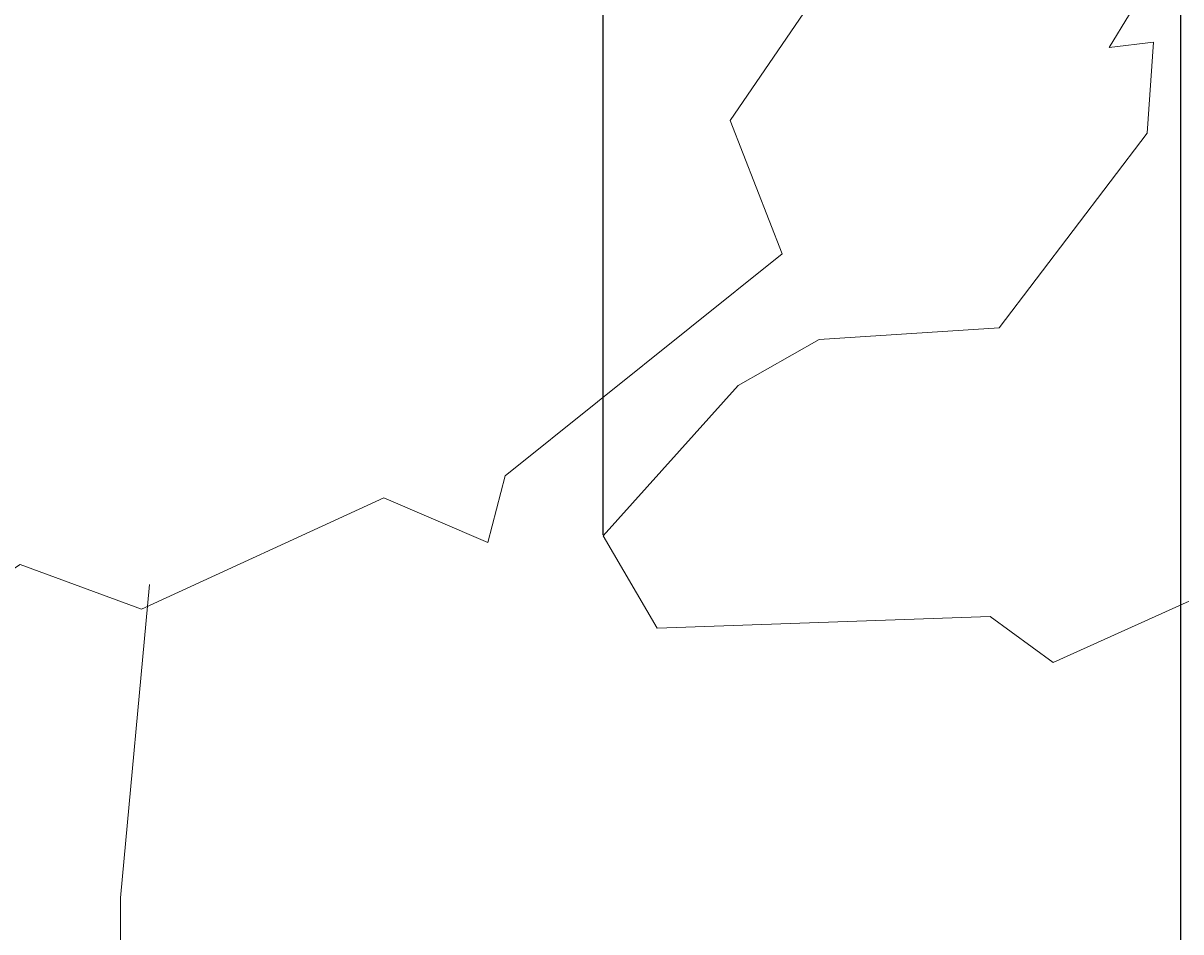
# Model space of a CAD drawing. Units: inches. Extents: x -26 to 776, y -22 to 650.
# Tile 44 of 62: x 506 to 584, y 40 to 102. Entities that reach past the tile are written whole.
import ezdxf

# ---------------------------------------------------------------- set-up
doc = ezdxf.new("R2010")
doc.units = ezdxf.units.IN
doc.header["$MEASUREMENT"] = 0
doc.layers.add('A-ANNO-DIMS', color=2, linetype='Continuous', lineweight=18)
doc.layers.add('L-PLNT-TREE', color=94, linetype='Continuous', lineweight=18)
doc.styles.get("Standard").update_dxf_attribs({"font": 'arial.ttf'})
doc.dimstyles.get("Standard").update_dxf_attribs({"dimtxt": 0.5625, "dimasz": 0.18, "dimexe": 0.18, "dimexo": 0.0625, "dimgap": 0.09, "dimtad": 0, "dimtih": 1, "dimtoh": 1, "dimdec": 4, "dimzin": 0, "dimdsep": 46, "dimlunit": 4, "dimtxsty": 'Standard', "dimcen": 0.09, "dimadec": 0, "dimazin": 0, "dimtfac": 1, "dimtdec": 4, "dimtofl": 0, "dimtmove": 0, "dimatfit": 3, "dimfxl": 1, "dimtolj": 1, "dimtzin": 0, "dimarcsym": 0})

# ---------------------------------------------------------------- blocks, each defined once
blk = doc.blocks.new('Tree - type 3 evergreen elevation')
blk.add_lwpolyline([(-41.4085, 64.6985), (-44.3346, 59.8898), (-42.2089, 60.1377), (-42.5159, 55.7849), (-49.6039, 46.4502), (-58.2307, 45.8972), (-62.1127, 43.6853), (-68.5828, 36.4966), (-65.9947, 32.0727), (-50.0352, 32.6257), (-47.0159, 30.4138), (-39.6831, 33.7317), (-34.507, 22.6721), (-32.3504, 22.6721), (-22.4296, 34.8376), (-19.4102, 36.4966), (-17.2536, 33.7317), (-17.2536, 29.8608), (-13.8028, 28.7549), (-9.0581, 28.7549), (-7.3328, 32.6257), (-1.7254, 35.3906), (3.8821, 35.9436)])
blk = doc.blocks.new('Tree - type 2 deciduous elevation')
for points in [[(-30.36, 44.975), (-31.51, 36.128), (-26.334, 36.865), (-23.459, 39.814), (-18.283, 36.128), (-20.008, 33.178), (-14.832, 31.704), (-11.956, 33.178), (-12.531, 27.28), (-6.205, 22.856), (-3.905, 24.331), (0.121, 22.856), (8.173, 26.543), (11.624, 25.068), (12.199, 27.28), (21.4, 34.653), (19.675, 39.077), (23.701, 44.975)], [(0.387, 23.669), (-0.576, 13.271), (-0.576, 3.686), (0, 0)]]:
    blk.add_lwpolyline(points)
blk = doc.blocks.new('*D13')
at = {"layer": 'A-ANNO-DIMS', "color": 0, "lineweight": -2, "transparency": 16777216}
for p, q in [((738.75, 50.786), (738.75, -21.315)), ((11.107, 15.42), (11.107, -21.315)), ((11.287, -21.135), (373.892, -21.135)), ((738.57, -21.135), (375.965, -21.135))]:
    blk.add_line(p, q, dxfattribs=at)
at = {"layer": 'A-ANNO-DIMS', "color": 0, "transparency": 16777216}
for points in [[(11.287, -21.105), (11.287, -21.165), (11.107, -21.135)], [(738.57, -21.105), (738.57, -21.165), (738.75, -21.135)]]:
    blk.add_solid(points, dxfattribs=at)
at = {"layer": 'Defpoints', "color": 0, "transparency": 16777216}
for p in [(738.75, 50.848), (11.107, 15.482), (738.75, -21.135)]:
    blk.add_point(p, dxfattribs=at)
at = {"layer": 'A-ANNO-DIMS', "color": 0, "transparency": 16777216, "insert": (374.929, -21.135), "char_height": 0.5625, "attachment_point": 5}
blk.add_mtext('\\A1;727.6', dxfattribs=at)
blk = doc.blocks.new('*D20')
at = {"layer": 'A-ANNO-DIMS', "color": 0, "lineweight": -2, "transparency": 16777216}
for p, q in [((425.806, 455.472), (775.335, 455.472)), ((775.155, 455.292), (775.155, 235.854)), ((775.155, 15.662), (775.155, 235.1)), ((425.806, 15.482), (775.335, 15.482))]:
    blk.add_line(p, q, dxfattribs=at)
at = {"layer": 'A-ANNO-DIMS', "color": 0, "transparency": 16777216}
for points in [[(775.125, 455.292), (775.185, 455.292), (775.155, 455.472)], [(775.125, 15.662), (775.185, 15.662), (775.155, 15.482)]]:
    blk.add_solid(points, dxfattribs=at)
at = {"layer": 'Defpoints', "color": 0, "transparency": 16777216}
for p in [(425.743, 455.472), (775.155, 455.472), (425.743, 15.482)]:
    blk.add_point(p, dxfattribs=at)
at = {"layer": 'A-ANNO-DIMS', "color": 0, "transparency": 16777216, "insert": (775.155, 235.477), "char_height": 0.5625, "attachment_point": 5}
blk.add_mtext('\\A1;440', dxfattribs=at)
blk = doc.blocks.new('*D30')
at = {"layer": 'A-ANNO-DIMS', "color": 0, "lineweight": -2, "transparency": 16777216}
for p, q in [((280.68, 144.836), (775.335, 144.836)), ((775.155, 144.656), (775.155, 86.007)), ((775.155, 26.604), (775.155, 85.253)), ((280.68, 26.424), (775.335, 26.424))]:
    blk.add_line(p, q, dxfattribs=at)
at = {"layer": 'A-ANNO-DIMS', "color": 0, "transparency": 16777216}
for points in [[(775.125, 144.656), (775.185, 144.656), (775.155, 144.836)], [(775.125, 26.604), (775.185, 26.604), (775.155, 26.424)]]:
    blk.add_solid(points, dxfattribs=at)
at = {"layer": 'Defpoints', "color": 0, "transparency": 16777216}
for p in [(280.617, 144.836), (775.155, 144.836), (280.617, 26.424)]:
    blk.add_point(p, dxfattribs=at)
at = {"layer": 'A-ANNO-DIMS', "color": 0, "transparency": 16777216, "insert": (775.155, 85.63), "char_height": 0.5625, "attachment_point": 5}
blk.add_mtext('\\A1;118.41', dxfattribs=at)
blk = doc.blocks.new('*D45')
at = {"layer": 'A-ANNO-DIMS', "color": 0, "lineweight": -2, "transparency": 16777216}
for p, q in [((507.738, 408.639), (775.335, 408.639)), ((775.155, 408.459), (775.155, 212.438)), ((775.155, 15.662), (775.155, 211.683)), ((585.998, 15.482), (775.335, 15.482))]:
    blk.add_line(p, q, dxfattribs=at)
at = {"layer": 'A-ANNO-DIMS', "color": 0, "transparency": 16777216}
for points in [[(775.125, 408.459), (775.185, 408.459), (775.155, 408.639)], [(775.125, 15.662), (775.185, 15.662), (775.155, 15.482)]]:
    blk.add_solid(points, dxfattribs=at)
at = {"layer": 'Defpoints', "color": 0, "transparency": 16777216}
for p in [(507.676, 408.639), (775.155, 408.639), (585.935, 15.482)]:
    blk.add_point(p, dxfattribs=at)
at = {"layer": 'A-ANNO-DIMS', "color": 0, "transparency": 16777216, "insert": (775.155, 212.061), "char_height": 0.5625, "attachment_point": 5}
blk.add_mtext('\\A1;393.16', dxfattribs=at)
blk = doc.blocks.new('*D47')
at = {"layer": 'A-ANNO-DIMS', "color": 0, "lineweight": -2, "transparency": 16777216}
for p, q in [((584.343, 199.901), (584.343, -21.315)), ((428.648, 180.243), (428.648, -21.315)), ((428.828, -21.135), (505.483, -21.135)), ((584.163, -21.135), (507.508, -21.135))]:
    blk.add_line(p, q, dxfattribs=at)
at = {"layer": 'A-ANNO-DIMS', "color": 0, "transparency": 16777216}
for points in [[(428.828, -21.105), (428.828, -21.165), (428.648, -21.135)], [(584.163, -21.105), (584.163, -21.165), (584.343, -21.135)]]:
    blk.add_solid(points, dxfattribs=at)
at = {"layer": 'Defpoints', "color": 0, "transparency": 16777216}
for p in [(584.343, 199.963), (428.648, 180.305), (584.343, -21.135)]:
    blk.add_point(p, dxfattribs=at)
at = {"layer": 'A-ANNO-DIMS', "color": 0, "transparency": 16777216, "insert": (506.496, -21.135), "char_height": 0.5625, "attachment_point": 5}
blk.add_mtext('\\A1;155.7', dxfattribs=at)
blk = doc.blocks.new('*D48')
at = {"layer": 'A-ANNO-DIMS', "color": 0, "lineweight": -2, "transparency": 16777216}
for p, q in [((545.033, 67.415), (545.033, 649.856)), ((738.75, 50.911), (738.75, 649.856)), ((545.213, 649.676), (640.879, 649.676)), ((738.57, 649.676), (642.904, 649.676))]:
    blk.add_line(p, q, dxfattribs=at)
at = {"layer": 'A-ANNO-DIMS', "color": 0, "transparency": 16777216}
for points in [[(545.213, 649.706), (545.213, 649.646), (545.033, 649.676)], [(738.57, 649.706), (738.57, 649.646), (738.75, 649.676)]]:
    blk.add_solid(points, dxfattribs=at)
at = {"layer": 'Defpoints', "color": 0, "transparency": 16777216}
for p in [(738.75, 649.676), (545.033, 67.352), (738.75, 50.848)]:
    blk.add_point(p, dxfattribs=at)
at = {"layer": 'A-ANNO-DIMS', "color": 0, "transparency": 16777216, "insert": (641.892, 649.676), "char_height": 0.5625, "attachment_point": 5}
blk.add_mtext('\\A1;193.7', dxfattribs=at)

msp = doc.modelspace()

# ---------------------------------------------------------------- block references
at = {"layer": 'L-PLNT-TREE'}
for name, p, xscale, yscale, zscale in [('Tree - type 2 deciduous elevation', (513.3241, 15.4824), 2.050905272406618, 2.050905272406618, 2.050905272406618), ('Tree - type 3 evergreen elevation', (642.5048, 15.4824), 1.421226385586178, 1.421226385586178, 1.421226385586178)]:
    msp.add_blockref(name, p, dxfattribs=dict(at, xscale=xscale, yscale=yscale, zscale=zscale))

# ---------------------------------------------------------------- dimensions: what is measured, and where the dimension line sits
at = {"layer": 'A-ANNO-DIMS'}
for base, p1, p2, picture, middle in [((738.7503, 649.6763), (545.0331, 67.3523), (738.7503, 50.8482), '*D48', (641.8917, 649.6763)), ((584.3428, -21.1349), (428.6484, 180.3054), (584.3428, 199.9634), '*D47', (506.4956, -21.1349)), ((738.7503, -21.1349), (11.1074, 15.4824), (738.7503, 50.8482), '*D13', (374.9289, -21.1349))]:
    dim = msp.add_linear_dim(base=base, p1=p1, p2=p2, dimstyle='Standard', override={"dimdec": 1, "dimlfac": 1, "dimrnd": 0, "dimzin": 0, "dimdsep": 46, "dimlunit": 2}, dxfattribs=at)
    dim.commit()
    dim.dimension.update_dxf_attribs({"geometry": picture, "text_midpoint": middle})
for base, p1, p2, override, picture, middle in [((775.1553, 455.4717), (425.7434, 15.4824), (425.7434, 455.4717), {"dimdec": 0, "dimlfac": 1, "dimrnd": 0, "dimzin": 0, "dimdsep": 46, "dimlunit": 2}, '*D20', (775.1553, 235.477)), ((775.1553, 408.6389), (585.9354, 15.4824), (507.6759, 408.6389), {"dimdec": 2, "dimlfac": 1, "dimrnd": 0, "dimzin": 0, "dimdsep": 46, "dimlunit": 2}, '*D45', (775.1553, 212.0606)), ((775.1553, 144.8359), (280.6173, 26.4239), (280.6173, 144.8359), {"dimdec": 2, "dimlfac": 1, "dimrnd": 0, "dimzin": 0, "dimdsep": 46, "dimlunit": 2}, '*D30', (775.1553, 85.6299))]:
    dim = msp.add_linear_dim(base=base, p1=p1, p2=p2, angle=90, dimstyle='Standard', override=override, dxfattribs=at)
    dim.commit()
    dim.dimension.update_dxf_attribs({"geometry": picture, "text_midpoint": middle})

doc.saveas('drawing.dxf')
